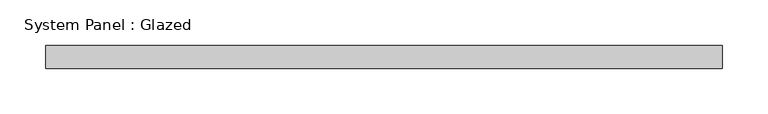
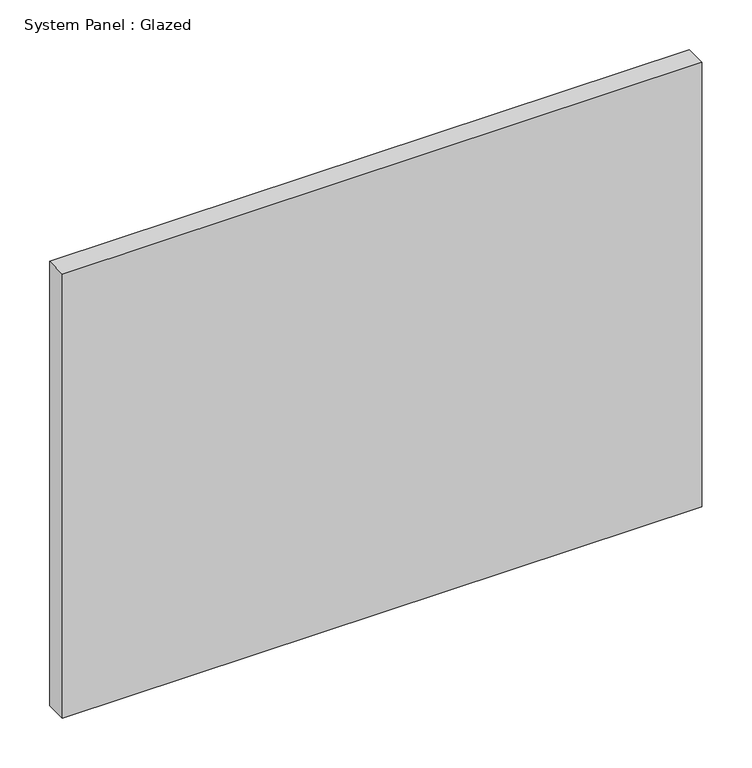
"""IFC4 building model written with IfcOpenShell, lengths in millimetres: plate geometry, System Panel : Glazed."""

from ifc_helpers import new_model, si_unit, origin, origin_with_axes, place, context, project, spatial, polyline, outline, extrude, source, transform, mapped, element, save


def system_panel_glazed_fea38f3a(model_context):
    return source(origin(), model_context, "Body", "SweptSolid", [
        extrude(outline(polyline([(371.475, 19.05), (-371.475, 19.05), (-371.475, 44.45), (371.475, 44.45), (371.475, 19.05)])), origin_with_axes(), (0.0, 0.0, 1.0), 545.6538352),
    ])


if __name__ == "__main__":
    model = new_model("IFC4")
    model_context = context("Model", 3, world=origin())
    ifc_project = project(units=[si_unit("LENGTHUNIT", "METRE", prefix="MILLI")], contexts=[model_context])
    site = spatial("IfcSite", under=ifc_project)
    building = spatial("IfcBuilding", under=site)
    placement = place(None, origin())
    system_panel_glazed_shape = system_panel_glazed_fea38f3a(model_context)
    element("IfcPlate", 1, ObjectType="System Panel : Glazed", at=placement, inside=building, context=model_context, shape_type="MappedRepresentation", body=[
        mapped(system_panel_glazed_shape, transform((0.0, 0.0, 0.0), x_axis=(1.0, 0.0, 0.0), y_axis=(0.0, 1.0, 0.0), z_axis=(0.0, 0.0, 1.0))),
    ])
    save(model, "model.ifc")

# Revit data of these elements
# Type "System Panel : Glazed"
#   Construction Type Id = "GSP4R"
#   Analytic Construction = "1/8 in Pilkington single glazing"
#   Visual Light Transmittance = 0.9
#   Solar Heat Gain Coefficient = 0.86
#   Heat Transfer Coefficient (U) = 1.18115 BTU/(h·ft²·°F)
#   Define Thermal Properties by = 1
# Element 1 (IfcPlate, "System Panel : Glazed")
#   Materials on its faces: "Glass"
# Materials
#   "Glass": class "Glass", colour RGB 0 128 192, transparency 0.75, Description = "Soda Lime Glass", Cost = 0
